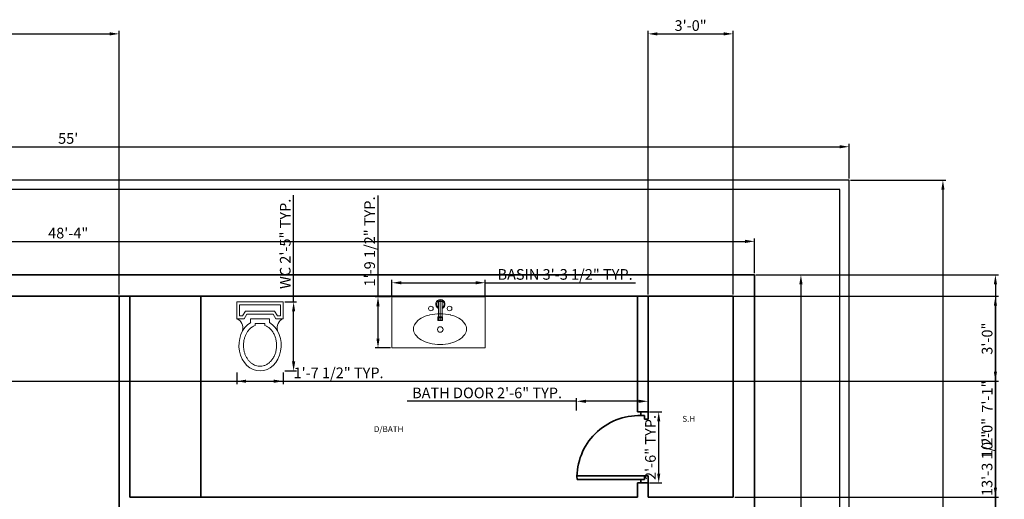
# Model space of a CAD drawing. Units: inches. Extents: x 1239 to 2276906, y 2273 to 321338.
# Tile 19 of 23: x 1620 to 2036, y 3411 to 3614. Entities that reach past the tile are written whole.
import ezdxf

# ---------------------------------------------------------------- set-up
doc = ezdxf.new("R2010")
doc.units = ezdxf.units.IN
for name, color, linetype, lineweight in [('A-ANNO-DIMS', 2, 'Continuous', 18), ('A-AREA-IDEN', 7, 'Continuous', 18), ('A-FLOR-FIXT', 9, 'Continuous', 18), ('C-PROP', 7, 'Continuous', 25), ('DOOR', 1, 'Continuous', 25), ('wall', 7, 'Continuous', 35)]:
    doc.layers.add(name, color=color, linetype=linetype, lineweight=lineweight)
doc.styles.get("Standard").update_dxf_attribs({"font": 'arial.ttf'})
doc.dimstyles.new('ISO-25', dxfattribs={"dimtxt": 4.5, "dimasz": 4, "dimexe": 1.25, "dimexo": 0.625, "dimtad": 1, "dimdec": 1, "dimlunit": 3, "dimtxsty": 'Standard', "dimcen": 2.5, "dimadec": 0, "dimazin": 0, "dimtfac": 1, "dimtdec": 1, "dimtmove": 0, "dimatfit": 3, "dimfxl": 1, "dimarcsym": 0})

# ---------------------------------------------------------------- blocks, each defined once
blk = doc.blocks.new('new block')
for p, q in [((1.5, 1.5), (1.5, 30)), ((3, 0), (3, 30)), ((0, 3), (0, 0)), ((1.5, 3), (0, 3)), ((0, 0), (3, 0)), ((1.5, 1.5), (1.5, 3)), ((3, 1.5), (1.5, 1.5)), ((3, 0), (3, 1.5)), ((27, 0), (27, 1.5)), ((27, 1.5), (28.5, 1.5)), ((30, 0), (27, 0)), ((28.5, 1.5), (28.5, 3)), ((28.5, 3), (30, 3)), ((30, 3), (30, 0))]:
    blk.add_line(p, q)
blk.add_arc((2.25, 3.75), 26.26, 358.3634, 91.6366)
blk = doc.blocks.new('2.6door')
at = {"layer": 'wall'}
blk.add_blockref('new block', (0, 0), dxfattribs=at)
blk = doc.blocks.new('A$C7C8779AE')
for p, q in [((0, 0.74), (0, 0.56)), ((0.5, 0.74), (0, 0.74)), ((0.5, 0.56), (0.5, 0.74)), ((0.47, 0.71), (0.03, 0.71)), ((0.03, 0.71), (0.03, 0.59)), ((0.093, 0.64), (0.063, 0.59)), ((0.093, 0.64), (0.407, 0.64)), ((0.437, 0.59), (0.407, 0.64)), ((0.47, 0.59), (0.47, 0.71)), ((0, 0.56), (0.08, 0.56)), ((0.03, 0.59), (0.063, 0.59)), ((0.11, 0.61), (0.08, 0.56)), ((0.11, 0.61), (0.39, 0.61)), ((0.15, 0.557), (0.15, 0.52)), ((0.15, 0.557), (0.351, 0.557)), ((0.351, 0.557), (0.351, 0.52)), ((0.42, 0.56), (0.39, 0.61)), ((0.42, 0.56), (0.5, 0.56)), ((0.437, 0.59), (0.47, 0.59)), ((0.2, 0.507), (0.2, 0.488)), ((0.2, 0.507), (0.301, 0.507)), ((0.301, 0.507), (0.301, 0.488))]:
    blk.add_line(p, q)
for centre, start, end in [((-0.039, 0.461), 344.642, 68.7339), ((0.539, 0.461), 111.2661, 195.358)]:
    blk.add_arc(centre, 0.106, start, end)
blk.add_ellipse((0.251, 0.274), major_axis=(0, 0.274), ratio=0.828948, start_param=0.459479, end_param=5.823706)
blk.add_open_spline([(0.2, 0.488), (0.17, 0.474), (0.164, 0.47), (0.151, 0.46), (0.144, 0.454), (0.13, 0.439), (0.123, 0.431), (0.111, 0.413), (0.106, 0.404), (0.096, 0.384), (0.091, 0.373), (0.084, 0.352), (0.081, 0.34), (0.076, 0.317), (0.075, 0.305), (0.073, 0.282), (0.073, 0.27), (0.074, 0.246), (0.076, 0.234), (0.08, 0.211), (0.083, 0.2), (0.09, 0.178), (0.095, 0.167), (0.104, 0.147), (0.11, 0.138), (0.122, 0.12), (0.128, 0.112), (0.142, 0.097), (0.149, 0.09), (0.165, 0.078), (0.173, 0.073), (0.189, 0.064), (0.197, 0.06), (0.214, 0.055), (0.222, 0.053), (0.239, 0.05), (0.248, 0.05), (0.266, 0.051), (0.276, 0.052), (0.296, 0.057), (0.306, 0.061), (0.325, 0.071), (0.335, 0.077), (0.353, 0.091), (0.361, 0.099), (0.377, 0.117), (0.384, 0.127), (0.398, 0.149), (0.404, 0.161), (0.414, 0.185), (0.418, 0.198), (0.424, 0.225), (0.426, 0.239), (0.428, 0.267), (0.428, 0.281), (0.426, 0.309), (0.424, 0.323), (0.418, 0.349), (0.414, 0.363), (0.404, 0.387), (0.398, 0.399), (0.385, 0.421), (0.378, 0.431), (0.362, 0.449), (0.353, 0.458), (0.338, 0.469), (0.332, 0.474), (0.301, 0.488)], degree=3, knots=[0.459479, 0.459479, 0.459479, 0.459479, 0.567422, 0.567422, 0.720865, 0.720865, 0.874307, 0.874307, 1.02775, 1.02775, 1.181192, 1.181192, 1.334635, 1.334635, 1.488077, 1.488077, 1.64152, 1.64152, 1.794963, 1.794963, 1.948405, 1.948405, 2.101848, 2.101848, 2.25529, 2.25529, 2.408733, 2.408733, 2.562175, 2.562175, 2.715618, 2.715618, 2.86906, 2.86906, 3.022503, 3.022503, 3.175946, 3.175946, 3.356457, 3.356457, 3.536968, 3.536968, 3.717479, 3.717479, 3.89799, 3.89799, 4.078501, 4.078501, 4.259012, 4.259012, 4.439523, 4.439523, 4.620035, 4.620035, 4.800546, 4.800546, 4.981057, 4.981057, 5.161568, 5.161568, 5.342079, 5.342079, 5.52259, 5.52259, 5.703101, 5.703101, 5.823706, 5.823706, 5.823706, 5.823706])
blk = doc.blocks.new('A$C50A015BB')
for p, q in [((0, 0.55), (1, 0.55)), ((0, 0.55), (0, 0)), ((1, 0.55), (1, 0)), ((0.498, 0.5), (0.538, 0.5)), ((0.498, 0.5), (0.498, 0.3)), ((0.518, 0.5), (0.518, 0.3)), ((0.538, 0.5), (0.538, 0.3)), ((0.493, 0.335), (0.493, 0.295)), ((0.493, 0.335), (0.543, 0.335)), ((0.498, 0.325), (0.538, 0.325)), ((0.543, 0.335), (0.543, 0.295)), ((0.493, 0.295), (0.543, 0.295)), ((0.498, 0.3), (0.538, 0.3)), ((0, 0), (1, 0)), ((0, 0), (1, 0))]:
    blk.add_line(p, q)
for centre, radius in [((0.418, 0.424), 0.025), ((0.618, 0.424), 0.025), ((0.518, 0.198), 0.0298)]:
    blk.add_circle(centre, radius)
for centre, radius, start, end in [((0.52, 0.47), 0.0497, 291.7425, 244.2331), ((0.52, 0.47), 0.0397, 297.632, 237.0256), ((0.418, 0.14), 0.208, 120.0686, 144.4178), ((0.477, 0.038), 0.325, 103.4853, 120.0686), ((0.516, -0.123), 0.491, 90, 103.4853), ((0.516, -0.123), 0.491, 76.5147, 90), ((0.554, 0.038), 0.325, 59.9314, 76.5147), ((0.613, 0.14), 0.208, 35.5822, 59.9314), ((0.33, 0.203), 0.0991, 144.4178, 180), ((0.702, 0.203), 0.0991, 0, 35.5822), ((0.33, 0.203), 0.0991, 180, 215.5822), ((0.418, 0.267), 0.208, 215.5822, 239.9314), ((0.613, 0.267), 0.208, 300.0686, 324.4178), ((0.702, 0.203), 0.0991, 324.4178, 0), ((0.477, 0.368), 0.325, 239.9314, 256.5147), ((0.516, 0.529), 0.491, 256.5147, 270), ((0.516, 0.529), 0.491, 270, 283.4853), ((0.554, 0.368), 0.325, 283.4853, 300.0686)]:
    blk.add_arc(centre, radius, start, end)
blk = doc.blocks.new('*D37')
at = {"layer": 'A-ANNO-DIMS', "color": 0, "lineweight": -2, "transparency": 16777216}
for p, q in [((1310.38, 3546.52), (1310.38, 3561.25)), ((1314.38, 3560), (1966.38, 3560)), ((1970.38, 3546.52), (1970.38, 3561.25))]:
    blk.add_line(p, q, dxfattribs=at)
at = {"layer": 'A-ANNO-DIMS', "color": 0, "transparency": 16777216}
for points in [[(1314.38, 3560.67), (1314.38, 3559.33), (1310.38, 3560)], [(1966.38, 3560.67), (1966.38, 3559.33), (1970.38, 3560)]]:
    blk.add_solid(points, dxfattribs=at)
at = {"layer": 'Defpoints', "color": 0, "transparency": 16777216}
for p in [(1970.38, 3560), (1310.38, 3545.9), (1970.38, 3545.9)]:
    blk.add_point(p, dxfattribs=at)
at = {"layer": 'A-ANNO-DIMS', "color": 0, "transparency": 16777216, "insert": (1640.38, 3562.91), "char_height": 4.5, "attachment_point": 5}
blk.add_mtext("55'", dxfattribs=at)
blk = doc.blocks.new('*D38')
at = {"layer": 'A-ANNO-DIMS', "color": 0, "lineweight": -2, "transparency": 16777216}
for p, q in [((1971.01, 3545.9), (2011.25, 3545.9)), ((2010, 3541.9), (2010, 2342.75)), ((1971.01, 2338.75), (2011.25, 2338.75))]:
    blk.add_line(p, q, dxfattribs=at)
at = {"layer": 'A-ANNO-DIMS', "color": 0, "transparency": 16777216}
for points in [[(2009.33, 3541.9), (2010.67, 3541.9), (2010, 3545.9)], [(2009.33, 2342.75), (2010.67, 2342.75), (2010, 2338.75)]]:
    blk.add_solid(points, dxfattribs=at)
at = {"layer": 'Defpoints', "color": 0, "transparency": 16777216}
for p in [(1970.38, 3545.9), (1970.38, 2338.75), (2010, 2338.75)]:
    blk.add_point(p, dxfattribs=at)
at = {"layer": 'A-ANNO-DIMS', "color": 0, "transparency": 16777216, "insert": (2007.08, 2942.32), "char_height": 4.5, "attachment_point": 5, "rotation": 90}
blk.add_mtext('100\'-7.2"', dxfattribs=at)
blk = doc.blocks.new('*D39')
at = {"layer": 'A-ANNO-DIMS', "color": 0, "lineweight": -2, "transparency": 16777216}
for p, q in [((1350.38, 3506.52), (1350.38, 3521.25)), ((1354.38, 3520), (1926.38, 3520)), ((1930.38, 3506.52), (1930.38, 3521.25))]:
    blk.add_line(p, q, dxfattribs=at)
at = {"layer": 'A-ANNO-DIMS', "color": 0, "transparency": 16777216}
for points in [[(1354.38, 3520.67), (1354.38, 3519.33), (1350.38, 3520)], [(1926.38, 3520.67), (1926.38, 3519.33), (1930.38, 3520)]]:
    blk.add_solid(points, dxfattribs=at)
at = {"layer": 'Defpoints', "color": 0, "transparency": 16777216}
for p in [(1930.38, 3520), (1350.38, 3505.9), (1930.38, 3505.9)]:
    blk.add_point(p, dxfattribs=at)
at = {"layer": 'A-ANNO-DIMS', "color": 0, "transparency": 16777216, "insert": (1640.38, 3522.92), "char_height": 4.5, "attachment_point": 5}
blk.add_mtext('48\'-4"', dxfattribs=at)
blk = doc.blocks.new('*D40')
at = {"layer": 'A-ANNO-DIMS', "color": 0, "lineweight": -2, "transparency": 16777216}
for p, q in [((1931.01, 3505.9), (1951.25, 3505.9)), ((1950, 3501.9), (1950, 2354)), ((1931.01, 2350), (1951.25, 2350))]:
    blk.add_line(p, q, dxfattribs=at)
at = {"layer": 'A-ANNO-DIMS', "color": 0, "transparency": 16777216}
for points in [[(1949.33, 3501.9), (1950.67, 3501.9), (1950, 3505.9)], [(1949.33, 2354), (1950.67, 2354), (1950, 2350)]]:
    blk.add_solid(points, dxfattribs=at)
at = {"layer": 'Defpoints', "color": 0, "transparency": 16777216}
for p in [(1930.38, 3505.9), (1930.38, 2350), (1950, 2350)]:
    blk.add_point(p, dxfattribs=at)
at = {"layer": 'A-ANNO-DIMS', "color": 0, "transparency": 16777216, "insert": (1947.08, 2927.95), "char_height": 4.5, "attachment_point": 5, "rotation": 90}
blk.add_mtext('96\'-3.9"', dxfattribs=at)
blk = doc.blocks.new('*D50')
at = {"layer": 'A-ANNO-DIMS', "color": 0, "lineweight": -2, "transparency": 16777216}
for p, q in [((1855.18, 3448.52), (1855.18, 3453.68)), ((1885.38, 3448.52), (1885.38, 3453.68)), ((1855.18, 3452.43), (1783.58, 3452.43)), ((1881.38, 3452.43), (1859.18, 3452.43))]:
    blk.add_line(p, q, dxfattribs=at)
at = {"layer": 'A-ANNO-DIMS', "color": 0, "transparency": 16777216}
for points in [[(1859.18, 3453.09), (1859.18, 3451.76), (1855.18, 3452.43)], [(1881.38, 3453.09), (1881.38, 3451.76), (1885.38, 3452.43)]]:
    blk.add_solid(points, dxfattribs=at)
at = {"layer": 'Defpoints', "color": 0, "transparency": 16777216}
for p in [(1855.18, 3452.43), (1855.18, 3447.9), (1885.38, 3447.9)]:
    blk.add_point(p, dxfattribs=at)
at = {"layer": 'A-ANNO-DIMS', "color": 0, "transparency": 16777216, "insert": (1817.38, 3455.38), "char_height": 4.5, "attachment_point": 5}
blk.add_mtext('BATH DOOR 2\'-6" TYP.', dxfattribs=at)
blk = doc.blocks.new('*D51')
at = {"layer": 'A-ANNO-DIMS', "color": 0, "lineweight": -2, "transparency": 16777216}
for p, q in [((1886.01, 3447.9), (1891.16, 3447.9)), ((1889.91, 3421.9), (1889.91, 3443.9)), ((1886.01, 3417.9), (1891.16, 3417.9))]:
    blk.add_line(p, q, dxfattribs=at)
at = {"layer": 'A-ANNO-DIMS', "color": 0, "transparency": 16777216}
for points in [[(1889.25, 3443.9), (1890.58, 3443.9), (1889.91, 3447.9)], [(1889.25, 3421.9), (1890.58, 3421.9), (1889.91, 3417.9)]]:
    blk.add_solid(points, dxfattribs=at)
at = {"layer": 'Defpoints', "color": 0, "transparency": 16777216}
for p in [(1885.38, 3447.9), (1889.91, 3447.9), (1885.38, 3417.9)]:
    blk.add_point(p, dxfattribs=at)
at = {"layer": 'A-ANNO-DIMS', "color": 0, "transparency": 16777216, "insert": (1886.99, 3432.9), "char_height": 4.5, "attachment_point": 5, "rotation": 90}
blk.add_mtext('2\'-6" TYP.', dxfattribs=at)
blk = doc.blocks.new('*D72')
at = {"layer": 'A-ANNO-DIMS', "color": 0, "lineweight": -2, "transparency": 16777216}
for p, q in [((1735.63, 3494.43), (1735.63, 3539.52)), ((1731.88, 3494.43), (1736.88, 3494.43)), ((1735.63, 3469.28), (1735.63, 3490.43)), ((1731.88, 3465.28), (1736.88, 3465.28))]:
    blk.add_line(p, q, dxfattribs=at)
at = {"layer": 'A-ANNO-DIMS', "color": 0, "transparency": 16777216}
for points in [[(1734.96, 3490.43), (1736.3, 3490.43), (1735.63, 3494.43)], [(1734.96, 3469.28), (1736.3, 3469.28), (1735.63, 3465.28)]]:
    blk.add_solid(points, dxfattribs=at)
at = {"layer": 'Defpoints', "color": 0, "transparency": 16777216}
for p in [(1731.26, 3494.43), (1735.63, 3494.43), (1731.26, 3465.28)]:
    blk.add_point(p, dxfattribs=at)
at = {"layer": 'A-ANNO-DIMS', "color": 0, "transparency": 16777216, "insert": (1732.68, 3518.97), "char_height": 4.5, "attachment_point": 5, "rotation": 90}
blk.add_mtext('WC 2\'-5" TYP.', dxfattribs=at)
blk = doc.blocks.new('*D73')
at = {"layer": 'A-ANNO-DIMS', "color": 0, "lineweight": -2, "transparency": 16777216}
for p, q in [((1711.57, 3464.65), (1711.57, 3459.66)), ((1731.26, 3464.65), (1731.26, 3459.66)), ((1715.57, 3460.91), (1727.26, 3460.91)), ((1731.26, 3460.91), (1774, 3460.91))]:
    blk.add_line(p, q, dxfattribs=at)
at = {"layer": 'A-ANNO-DIMS', "color": 0, "transparency": 16777216}
for points in [[(1715.57, 3461.57), (1715.57, 3460.24), (1711.57, 3460.91)], [(1727.26, 3461.57), (1727.26, 3460.24), (1731.26, 3460.91)]]:
    blk.add_solid(points, dxfattribs=at)
at = {"layer": 'Defpoints', "color": 0, "transparency": 16777216}
for p in [(1711.57, 3465.28), (1731.26, 3465.28), (1731.26, 3460.91)]:
    blk.add_point(p, dxfattribs=at)
at = {"layer": 'A-ANNO-DIMS', "color": 0, "transparency": 16777216, "insert": (1754.63, 3463.86), "char_height": 4.5, "attachment_point": 5}
blk.add_mtext('1\'-7 1/2" TYP.', dxfattribs=at)
blk = doc.blocks.new('*D74')
at = {"layer": 'A-ANNO-DIMS', "color": 0, "lineweight": -2, "transparency": 16777216}
for p, q in [((1777.19, 3497.23), (1777.19, 3503.76)), ((1816.56, 3497.23), (1816.56, 3503.76)), ((1781.19, 3502.51), (1812.56, 3502.51)), ((1816.56, 3502.51), (1880.14, 3502.51))]:
    blk.add_line(p, q, dxfattribs=at)
at = {"layer": 'A-ANNO-DIMS', "color": 0, "transparency": 16777216}
for points in [[(1781.19, 3503.18), (1781.19, 3501.84), (1777.19, 3502.51)], [(1812.56, 3503.18), (1812.56, 3501.84), (1816.56, 3502.51)]]:
    blk.add_solid(points, dxfattribs=at)
at = {"layer": 'Defpoints', "color": 0, "transparency": 16777216}
for p in [(1816.56, 3502.51), (1777.19, 3496.6), (1816.56, 3496.6)]:
    blk.add_point(p, dxfattribs=at)
at = {"layer": 'A-ANNO-DIMS', "color": 0, "transparency": 16777216, "insert": (1850.35, 3505.46), "char_height": 4.5, "attachment_point": 5}
blk.add_mtext('BASIN 3\'-3 1/2" TYP.', dxfattribs=at)
blk = doc.blocks.new('*D75')
at = {"layer": 'A-ANNO-DIMS', "color": 0, "lineweight": -2, "transparency": 16777216}
for p, q in [((1771.29, 3496.6), (1771.29, 3539.34)), ((1776.57, 3496.6), (1770.04, 3496.6)), ((1771.29, 3478.95), (1771.29, 3492.6)), ((1776.57, 3474.95), (1770.04, 3474.95))]:
    blk.add_line(p, q, dxfattribs=at)
at = {"layer": 'A-ANNO-DIMS', "color": 0, "transparency": 16777216}
for points in [[(1770.62, 3492.6), (1771.95, 3492.6), (1771.29, 3496.6)], [(1770.62, 3478.95), (1771.95, 3478.95), (1771.29, 3474.95)]]:
    blk.add_solid(points, dxfattribs=at)
at = {"layer": 'Defpoints', "color": 0, "transparency": 16777216}
for p in [(1771.29, 3496.6), (1777.19, 3496.6), (1777.19, 3474.95)]:
    blk.add_point(p, dxfattribs=at)
at = {"layer": 'A-ANNO-DIMS', "color": 0, "transparency": 16777216, "insert": (1768.34, 3519.97), "char_height": 4.5, "attachment_point": 5, "rotation": 90}
blk.add_mtext('1\'-9 1/2" TYP.', dxfattribs=at)
blk = doc.blocks.new('*D84')
at = {"layer": 'A-ANNO-DIMS', "color": 0, "lineweight": -2, "transparency": 16777216}
for p, q in [((1469.88, 3497.52), (1469.88, 3608.95)), ((1473.88, 3607.7), (1657.88, 3607.7)), ((1661.88, 3497.52), (1661.88, 3608.95))]:
    blk.add_line(p, q, dxfattribs=at)
at = {"layer": 'A-ANNO-DIMS', "color": 0, "transparency": 16777216}
for points in [[(1473.88, 3608.36), (1473.88, 3607.03), (1469.88, 3607.7)], [(1657.88, 3608.36), (1657.88, 3607.03), (1661.88, 3607.7)]]:
    blk.add_solid(points, dxfattribs=at)
at = {"layer": 'Defpoints', "color": 0, "transparency": 16777216}
for p in [(1661.88, 3607.7), (1469.88, 3496.9), (1661.88, 3496.9)]:
    blk.add_point(p, dxfattribs=at)
at = {"layer": 'A-ANNO-DIMS', "color": 0, "transparency": 16777216, "insert": (1565.88, 3610.62), "char_height": 4.5, "attachment_point": 5}
blk.add_mtext('16\'-0"', dxfattribs=at)
blk = doc.blocks.new('*D85')
at = {"layer": 'A-ANNO-DIMS', "color": 0, "lineweight": -2, "transparency": 16777216}
for p, q in [((1470.51, 3496.9), (2033.43, 3496.9)), ((2032.18, 3380.9), (2032.18, 3492.9)), ((1470.51, 3376.9), (2033.43, 3376.9))]:
    blk.add_line(p, q, dxfattribs=at)
at = {"layer": 'A-ANNO-DIMS', "color": 0, "transparency": 16777216}
for points in [[(2031.52, 3492.9), (2032.85, 3492.9), (2032.18, 3496.9)], [(2031.52, 3380.9), (2032.85, 3380.9), (2032.18, 3376.9)]]:
    blk.add_solid(points, dxfattribs=at)
at = {"layer": 'Defpoints', "color": 0, "transparency": 16777216}
for p in [(1469.88, 3496.9), (2032.18, 3496.9), (1469.88, 3376.9)]:
    blk.add_point(p, dxfattribs=at)
at = {"layer": 'A-ANNO-DIMS', "color": 0, "transparency": 16777216, "insert": (2029.26, 3436.9), "char_height": 4.5, "attachment_point": 5, "rotation": 90}
blk.add_mtext('10\'-0"', dxfattribs=at)
blk = doc.blocks.new('*D86')
at = {"layer": 'A-ANNO-DIMS', "color": 0, "lineweight": -2, "transparency": 16777216}
for p, q in [((1885.38, 3497.52), (1885.38, 3608.95)), ((1889.38, 3607.7), (1917.38, 3607.7)), ((1921.38, 3497.52), (1921.38, 3608.95))]:
    blk.add_line(p, q, dxfattribs=at)
at = {"layer": 'A-ANNO-DIMS', "color": 0, "transparency": 16777216}
for points in [[(1889.38, 3608.36), (1889.38, 3607.03), (1885.38, 3607.7)], [(1917.38, 3608.36), (1917.38, 3607.03), (1921.38, 3607.7)]]:
    blk.add_solid(points, dxfattribs=at)
at = {"layer": 'Defpoints', "color": 0, "transparency": 16777216}
for p in [(1921.38, 3607.7), (1885.38, 3496.9), (1921.38, 3496.9)]:
    blk.add_point(p, dxfattribs=at)
at = {"layer": 'A-ANNO-DIMS', "color": 0, "transparency": 16777216, "insert": (1903.38, 3610.62), "char_height": 4.5, "attachment_point": 5}
blk.add_mtext('3\'-0"', dxfattribs=at)
blk = doc.blocks.new('*D108')
at = {"layer": 'A-ANNO-DIMS', "color": 0, "lineweight": -2, "transparency": 16777216}
for p, q in [((1931.01, 3505.9), (2033.43, 3505.9)), ((2032.18, 3501.9), (2032.18, 3350.46)), ((1931.01, 3346.46), (2033.43, 3346.46))]:
    blk.add_line(p, q, dxfattribs=at)
at = {"layer": 'A-ANNO-DIMS', "color": 0, "transparency": 16777216}
for points in [[(2031.52, 3501.9), (2032.85, 3501.9), (2032.18, 3505.9)], [(2031.52, 3350.46), (2032.85, 3350.46), (2032.18, 3346.46)]]:
    blk.add_solid(points, dxfattribs=at)
at = {"layer": 'Defpoints', "color": 0, "transparency": 16777216}
for p in [(1930.38, 3505.9), (1930.38, 3346.46), (2032.18, 3346.46)]:
    blk.add_point(p, dxfattribs=at)
at = {"layer": 'A-ANNO-DIMS', "color": 0, "transparency": 16777216, "insert": (2029.23, 3426.18), "char_height": 4.5, "attachment_point": 5, "rotation": 90}
blk.add_mtext('13\'-3 1/2"', dxfattribs=at)
blk = doc.blocks.new('*D116')
at = {"layer": 'A-ANNO-DIMS', "color": 0, "lineweight": -2, "transparency": 16777216}
for p, q in [((1360.01, 3496.9), (2033.43, 3496.9)), ((2032.18, 3464.9), (2032.18, 3492.9)), ((1360.01, 3460.9), (2033.43, 3460.9))]:
    blk.add_line(p, q, dxfattribs=at)
at = {"layer": 'A-ANNO-DIMS', "color": 0, "transparency": 16777216}
for points in [[(2031.52, 3492.9), (2032.85, 3492.9), (2032.18, 3496.9)], [(2031.52, 3464.9), (2032.85, 3464.9), (2032.18, 3460.9)]]:
    blk.add_solid(points, dxfattribs=at)
at = {"layer": 'Defpoints', "color": 0, "transparency": 16777216}
for p in [(1359.38, 3496.9), (2032.18, 3496.9), (1359.38, 3460.9)]:
    blk.add_point(p, dxfattribs=at)
at = {"layer": 'A-ANNO-DIMS', "color": 0, "transparency": 16777216, "insert": (2029.26, 3478.9), "char_height": 4.5, "attachment_point": 5, "rotation": 90}
blk.add_mtext('3\'-0"', dxfattribs=at)
blk = doc.blocks.new('*D117')
at = {"layer": 'A-ANNO-DIMS', "color": 0, "lineweight": -2, "transparency": 16777216}
for p, q in [((1922.01, 3496.9), (2033.43, 3496.9)), ((2032.18, 3415.9), (2032.18, 3492.9)), ((1922.01, 3411.9), (2033.43, 3411.9))]:
    blk.add_line(p, q, dxfattribs=at)
at = {"layer": 'A-ANNO-DIMS', "color": 0, "transparency": 16777216}
for points in [[(2031.52, 3492.9), (2032.85, 3492.9), (2032.18, 3496.9)], [(2031.52, 3415.9), (2032.85, 3415.9), (2032.18, 3411.9)]]:
    blk.add_solid(points, dxfattribs=at)
at = {"layer": 'Defpoints', "color": 0, "transparency": 16777216}
for p in [(1921.38, 3496.9), (2032.18, 3496.9), (1921.38, 3411.9)]:
    blk.add_point(p, dxfattribs=at)
at = {"layer": 'A-ANNO-DIMS', "color": 0, "transparency": 16777216, "insert": (2029.3, 3454.4), "char_height": 4.5, "attachment_point": 5, "rotation": 90}
blk.add_mtext('7\'-1"', dxfattribs=at)

msp = doc.modelspace()

# ---------------------------------------------------------------- linework, layer by layer
at = {"layer": 'C-PROP'}
for points in [[(1970.38, 2345.9), (1970.38, 3545.9), (1310.38, 3545.9), (1310.38, 2345.9), (1644.79, 2345.9)], [(1966.38, 2349.9), (1966.38, 3541.9), (1314.38, 3541.9), (1314.38, 2607.52)]]:
    msp.add_lwpolyline(points, dxfattribs=at)
at = {"layer": 'wall'}
for p, q in [((1930.38, 3505.9), (1350.38, 3505.9)), ((1930.38, 2385.9), (1930.38, 3505.9)), ((1921.38, 3496.9), (1359.38, 3496.9)), ((1661.88, 3496.9), (1661.88, 3376.9)), ((1666.38, 3496.9), (1666.38, 3411.9)), ((1696.48, 3496.9), (1696.48, 3411.9)), ((1880.88, 3447.9), (1880.88, 3496.9)), ((1885.38, 3447.9), (1885.38, 3496.9)), ((1921.38, 3411.9), (1921.38, 3496.9)), ((1880.88, 3447.9), (1885.38, 3447.9)), ((1880.88, 3411.9), (1880.88, 3417.9)), ((1880.88, 3417.9), (1885.38, 3417.9)), ((1885.38, 3411.9), (1885.38, 3417.9)), ((1880.88, 3411.9), (1666.38, 3411.9)), ((1921.38, 3411.9), (1885.38, 3411.9))]:
    msp.add_line(p, q, dxfattribs=at)

# ---------------------------------------------------------------- block references
at = {"layer": 'A-FLOR-FIXT', "xscale": 39.37007874015748, "yscale": 39.37007874015748, "zscale": 39.37007874015748}
for name, p in [('A$C50A015BB', (1777.19, 3474.95)), ('A$C7C8779AE', (1711.57, 3465.28))]:
    msp.add_blockref(name, p, dxfattribs=at)
at = {"layer": 'DOOR', "rotation": 90}
msp.add_blockref('2.6door', (1885.38, 3417.9), dxfattribs=at)

# ---------------------------------------------------------------- texts
at = {"layer": 'A-AREA-IDEN', "char_height": 2.5, "attachment_point": 1}
for s, insert in [('S.H ', (1899.89, 3446.26)), ('D/BATH ', (1769.53, 3441.91))]:
    msp.add_mtext_dynamic_manual_height_columns(s, width=44.9462, gutter_width=12.5, heights=[0], dxfattribs=dict(at, insert=insert))

# ---------------------------------------------------------------- dimensions: what is measured, and where the dimension line sits
at = {"layer": 'A-ANNO-DIMS'}
for base, p1, p2, override, picture, middle in [((1661.88, 3607.7), (1469.88, 3496.9), (1661.88, 3496.9), {"dimdec": 1, "dimlfac": 1, "dimrnd": 0, "dimzin": 1, "dimdsep": 46, "dimlunit": 4, "dimfrac": 2}, '*D84', (1565.88, 3610.62)), ((1921.38, 3607.7), (1885.38, 3496.9), (1921.38, 3496.9), {"dimdec": 1, "dimlfac": 1, "dimrnd": 0, "dimzin": 1, "dimdsep": 46, "dimlunit": 4, "dimfrac": 2}, '*D86', (1903.38, 3610.62)), ((1970.38, 3560), (1310.38, 3545.9), (1970.38, 3545.9), {"dimclrd": 0, "dimclre": 0, "dimclrt": 0}, '*D37', (1640.38, 3562.91)), ((1930.38, 3520), (1350.38, 3505.9), (1930.38, 3505.9), {"dimclrd": 0, "dimclre": 0, "dimclrt": 0}, '*D39', (1640.38, 3522.92))]:
    dim = msp.add_linear_dim(base=base, p1=p1, p2=p2, dimstyle='ISO-25', override=override, dxfattribs=at)
    dim.commit()
    dim.dimension.update_dxf_attribs({"geometry": picture, "text_midpoint": middle})
for base, p1, p2, override, picture, middle in [((2010, 2338.7461), (1970.3833, 3545.8972), (1970.3833, 2338.7461), {"dimclrd": 0, "dimclre": 0, "dimclrt": 0}, '*D38', (2007.0774, 2942.3216)), ((1950, 2350), (1930.38, 3505.9), (1930.38, 2350), {"dimclrd": 0, "dimclre": 0, "dimclrt": 0}, '*D40', (1947.08, 2927.95)), ((2032.18, 3346.46), (1930.38, 3505.9), (1930.38, 3346.46), {"dimdec": 1, "dimlfac": 1, "dimrnd": 0, "dimzin": 1, "dimdsep": 46, "dimlunit": 4, "dimfrac": 2}, '*D108', (2029.23, 3426.18)), ((2032.18, 3496.9), (1359.38, 3460.9), (1359.38, 3496.9), {"dimdec": 1, "dimlfac": 1, "dimrnd": 0, "dimzin": 1, "dimdsep": 46, "dimlunit": 4, "dimfrac": 2}, '*D116', (2029.26, 3478.9)), ((2032.18, 3496.9), (1469.88, 3376.9), (1469.88, 3496.9), {"dimdec": 1, "dimlfac": 1, "dimrnd": 0, "dimzin": 1, "dimdsep": 46, "dimlunit": 4, "dimfrac": 2}, '*D85', (2029.26, 3436.9)), ((2032.18, 3496.9), (1921.38, 3411.9), (1921.38, 3496.9), {"dimdec": 1, "dimlfac": 1, "dimrnd": 0, "dimzin": 1, "dimdsep": 46, "dimlunit": 4, "dimfrac": 2}, '*D117', (2029.3, 3454.4))]:
    dim = msp.add_linear_dim(base=base, p1=p1, p2=p2, angle=90, dimstyle='ISO-25', override=override, dxfattribs=at)
    dim.commit()
    dim.dimension.update_dxf_attribs({"geometry": picture, "text_midpoint": middle})
for base, p1, p2, angle, text, picture, middle in [((1735.6311, 3494.4318), (1731.2583, 3465.2797), (1731.2583, 3494.4318), 90, 'WC <> TYP.', '*D72', (1732.6794, 3518.9737)), ((1771.2878, 3496.6029), (1777.1933, 3474.9494), (1777.1933, 3496.6029), 90, '<> TYP.', '*D75', (1768.336, 3519.9739)), ((1855.18, 3452.43), (1885.38, 3447.9), (1855.18, 3447.9), 180, 'BATH DOOR <> TYP.', '*D50', (1817.38, 3455.38)), ((1889.91, 3447.9), (1885.38, 3417.9), (1885.38, 3447.9), 90, '<> TYP.', '*D51', (1886.99, 3432.9))]:
    dim = msp.add_linear_dim(base=base, p1=p1, p2=p2, angle=angle, text=text, dimstyle='ISO-25', override={"dimdec": 1, "dimlfac": 1, "dimrnd": 0, "dimzin": 1, "dimdsep": 46, "dimlunit": 4, "dimfrac": 2}, dxfattribs=at)
    dim.commit()
    dim.dimension.update_dxf_attribs({"geometry": picture, "text_midpoint": middle})
for base, p1, p2, text, picture, middle in [((1816.56, 3502.51), (1777.19, 3496.6), (1816.56, 3496.6), 'BASIN <> TYP.', '*D74', (1850.35, 3505.46)), ((1731.26, 3460.91), (1711.57, 3465.28), (1731.26, 3465.28), '<> TYP.', '*D73', (1754.63, 3463.86))]:
    dim = msp.add_linear_dim(base=base, p1=p1, p2=p2, text=text, dimstyle='ISO-25', override={"dimdec": 1, "dimlfac": 1, "dimrnd": 0, "dimzin": 1, "dimdsep": 46, "dimlunit": 4, "dimfrac": 2}, dxfattribs=at)
    dim.commit()
    dim.dimension.update_dxf_attribs({"geometry": picture, "text_midpoint": middle})

doc.saveas('drawing.dxf')
